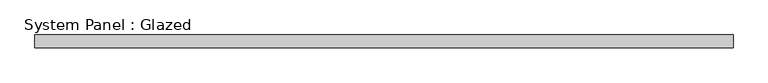
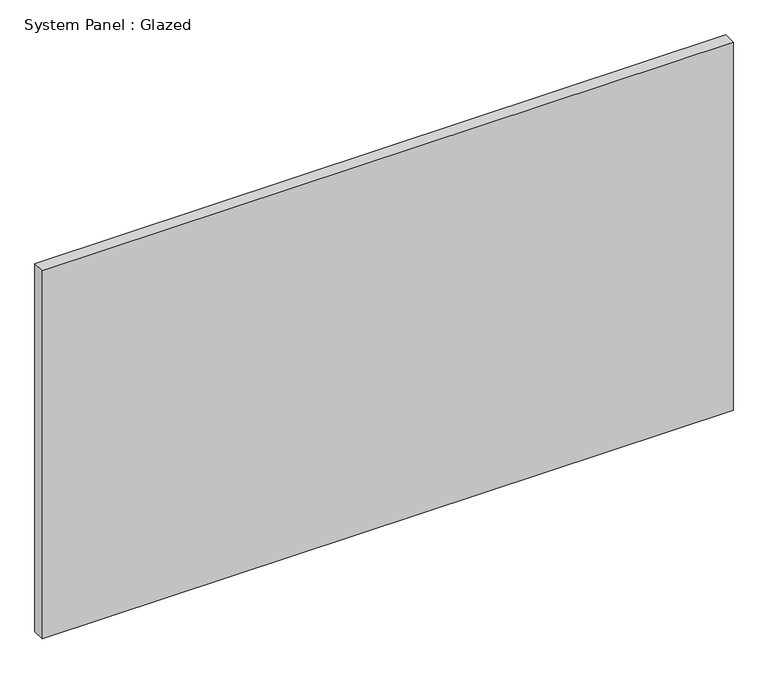
"""IFC4 building model written with IfcOpenShell, lengths in millimetres: plate geometry, System Panel : Glazed."""

from ifc_helpers import new_model, si_unit, origin, origin_with_axes, place, context, project, spatial, polyline, outline, extrude, source, transform, mapped, element, save


def system_panel_glazed_ff4fffb2(model_context):
    return source(origin(), model_context, "Body", "SweptSolid", [
        extrude(outline(polyline([(699.1185948, 19.05), (-699.1185948, 19.05), (-699.1185948, 44.45), (699.1185948, 44.45), (699.1185948, 19.05)])), origin_with_axes(), (0.0, 0.0, 1.0), 787.4),
    ])


if __name__ == "__main__":
    model = new_model("IFC4")
    model_context = context("Model", 3, world=origin())
    ifc_project = project(units=[si_unit("LENGTHUNIT", "METRE", prefix="MILLI")], contexts=[model_context])
    site = spatial("IfcSite", under=ifc_project)
    building = spatial("IfcBuilding", under=site)
    placement = place(None, origin())
    system_panel_glazed_shape = system_panel_glazed_ff4fffb2(model_context)
    element("IfcPlate", 1, ObjectType="System Panel : Glazed", at=placement, inside=building, context=model_context, shape_type="MappedRepresentation", body=[
        mapped(system_panel_glazed_shape, transform((0.0, 0.0, 0.0), x_axis=(1.0, 0.0, 0.0), y_axis=(0.0, 1.0, 0.0), z_axis=(0.0, 0.0, 1.0))),
    ])
    save(model, "model.ifc")

# Revit data of these elements
# Type "System Panel : Glazed"
#   Construction Type Id = "GSP4R"
#   Analytic Construction = "1/8 in Pilkington single glazing"
#   Visual Light Transmittance = 0.9
#   Solar Heat Gain Coefficient = 0.86
#   Heat Transfer Coefficient (U) = 1.18115 BTU/(h·ft²·°F)
#   Define Thermal Properties by = 1
# Element 1 (IfcPlate, "System Panel : Glazed")
#   Materials on its faces: "Glass"
# Materials
#   "Glass": class "Glass", colour RGB 0 128 192, transparency 0.75, Description = "Soda Lime Glass", Cost = 0
